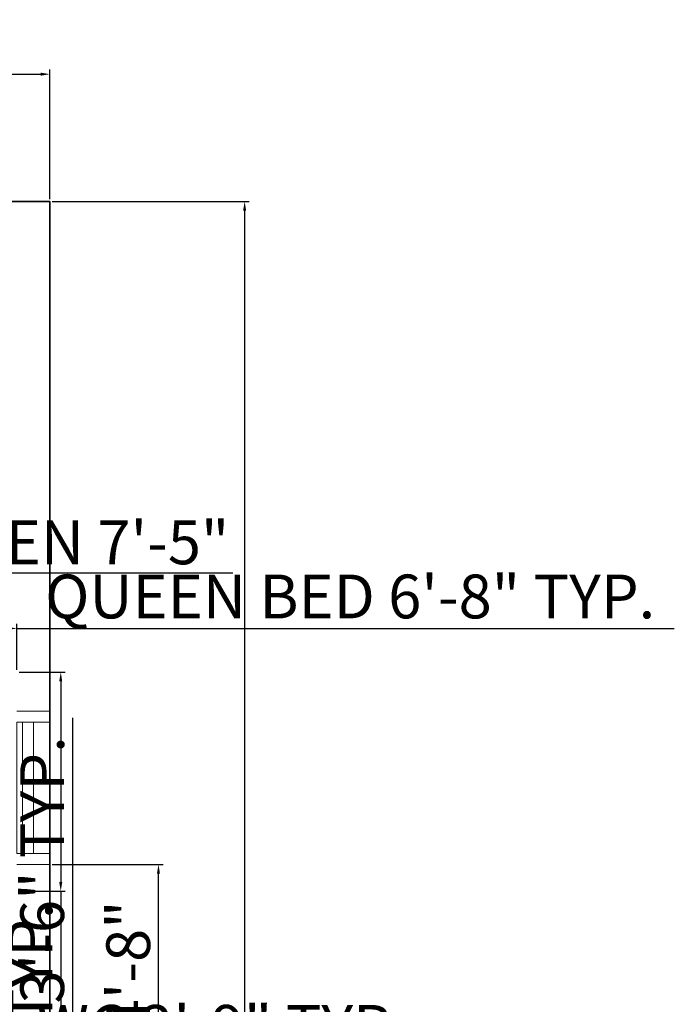
# Model space of a CAD drawing. Units: inches. Extents: x 2011 to 2548, y 530 to 1188.
# Tile 5 of 5: x 2368 to 2548, y 891 to 1161. Entities that reach past the tile are written whole.
import ezdxf

# ---------------------------------------------------------------- set-up
doc = ezdxf.new("R2010")
doc.units = ezdxf.units.IN
for name, color, linetype, lineweight in [('A-ANNO-DIMS', 2, 'Continuous', 18), ('A-GLAZ', 4, 'Continuous', 18), ('A-WALL', 7, 'Continuous', 35)]:
    doc.layers.add(name, color=color, linetype=linetype, lineweight=lineweight)
doc.styles.get("Standard").update_dxf_attribs({"font": 'arial.ttf'})
doc.dimstyles.new('ISO-25', dxfattribs={"dimtxt": 12, "dimasz": 2.5, "dimexe": 1.25, "dimexo": 0.625, "dimtad": 1, "dimdec": 1, "dimlunit": 3, "dimtxsty": 'Standard', "dimcen": 2.5, "dimadec": 0, "dimazin": 0, "dimtfac": 1, "dimtdec": 1, "dimtmove": 0, "dimatfit": 3, "dimfxl": 1, "dimarcsym": 0})

# ---------------------------------------------------------------- blocks, each defined once
blk = doc.blocks.new('*D12')
at = {"layer": 'A-ANNO-DIMS', "color": 0, "lineweight": -2, "transparency": 16777216}
for p, q in [((2076.53, 1111.98), (2076.53, 1147.49)), ((2376.53, 1111.98), (2376.53, 1147.49)), ((2079.03, 1146.24), (2374.03, 1146.24))]:
    blk.add_line(p, q, dxfattribs=at)
at = {"layer": 'A-ANNO-DIMS', "color": 0, "transparency": 16777216}
for points in [[(2079.03, 1146.66), (2079.03, 1145.82), (2076.53, 1146.24)], [(2374.03, 1146.66), (2374.03, 1145.82), (2376.53, 1146.24)]]:
    blk.add_solid(points, dxfattribs=at)
at = {"layer": 'Defpoints', "color": 0, "transparency": 16777216}
for p in [(2376.53, 1146.24), (2076.53, 1111.36), (2376.53, 1111.36)]:
    blk.add_point(p, dxfattribs=at)
at = {"layer": 'A-ANNO-DIMS', "color": 0, "transparency": 16777216, "insert": (2226.53, 1152.99), "char_height": 12, "attachment_point": 5}
blk.add_mtext("25'", dxfattribs=at)
blk = doc.blocks.new('*D13')
at = {"layer": 'A-ANNO-DIMS', "color": 0, "lineweight": -2, "transparency": 16777216}
for p, q in [((2377.15, 1111.36), (2431.21, 1111.36)), ((2429.96, 1108.86), (2429.96, 573.86)), ((2377.15, 571.36), (2431.21, 571.36))]:
    blk.add_line(p, q, dxfattribs=at)
at = {"layer": 'A-ANNO-DIMS', "color": 0, "transparency": 16777216}
for points in [[(2429.55, 1108.86), (2430.38, 1108.86), (2429.96, 1111.36)], [(2429.55, 573.86), (2430.38, 573.86), (2429.96, 571.36)]]:
    blk.add_solid(points, dxfattribs=at)
at = {"layer": 'Defpoints', "color": 0, "transparency": 16777216}
for p in [(2376.53, 1111.36), (2376.53, 571.36), (2429.96, 571.36)]:
    blk.add_point(p, dxfattribs=at)
at = {"layer": 'A-ANNO-DIMS', "color": 0, "transparency": 16777216, "insert": (2423.24, 841.36), "char_height": 12, "attachment_point": 5, "rotation": 90}
blk.add_mtext("45'", dxfattribs=at)
blk = doc.blocks.new('WIN-36IN')
for p, q in [((0, 42), (9, 42)), ((0, 3), (0, 39)), ((0, 39), (9, 39)), ((1.5, 39), (1.5, 3)), ((4.5, 39), (4.5, 3)), ((9, 39), (9, 3)), ((9, 3), (0, 3)), ((9, 0), (0, 0))]:
    blk.add_line(p, q)
blk = doc.blocks.new('*D17')
at = {"layer": 'A-ANNO-DIMS', "color": 0, "lineweight": -2, "transparency": 16777216}
for p, q in [((2382.83, 784.45), (2382.83, 969.85)), ((2377.15, 784.45), (2384.08, 784.45)), ((2382.83, 744.95), (2382.83, 781.95)), ((2377.15, 742.45), (2384.08, 742.45))]:
    blk.add_line(p, q, dxfattribs=at)
at = {"layer": 'A-ANNO-DIMS', "color": 0, "transparency": 16777216}
for points in [[(2382.41, 781.95), (2383.24, 781.95), (2382.83, 784.45)], [(2382.41, 744.95), (2383.24, 744.95), (2382.83, 742.45)]]:
    blk.add_solid(points, dxfattribs=at)
at = {"layer": 'Defpoints', "color": 0, "transparency": 16777216}
for p in [(2376.53, 784.45), (2382.83, 784.45), (2376.53, 742.45)]:
    blk.add_point(p, dxfattribs=at)
at = {"layer": 'A-ANNO-DIMS', "color": 0, "transparency": 16777216, "insert": (2375.99, 878.4), "char_height": 12, "attachment_point": 5, "rotation": 90}
blk.add_mtext('WINDOW W1 3\'-6" TYP.', dxfattribs=at)
blk = doc.blocks.new('*D23')
at = {"layer": 'A-ANNO-DIMS', "color": 0, "lineweight": -2, "transparency": 16777216}
for p, q in [((2334.48, 872.46), (2334.48, 878.04)), ((2367.53, 872.46), (2367.53, 878.04)), ((2336.98, 876.79), (2365.03, 876.79)), ((2367.53, 876.79), (2477.5, 876.79))]:
    blk.add_line(p, q, dxfattribs=at)
at = {"layer": 'A-ANNO-DIMS', "color": 0, "transparency": 16777216}
for points in [[(2336.98, 877.21), (2336.98, 876.38), (2334.48, 876.79)], [(2365.03, 877.21), (2365.03, 876.38), (2367.53, 876.79)]]:
    blk.add_solid(points, dxfattribs=at)
at = {"layer": 'Defpoints', "color": 0, "transparency": 16777216}
for p in [(2367.53, 876.79), (2334.48, 871.84), (2367.53, 871.84)]:
    blk.add_point(p, dxfattribs=at)
at = {"layer": 'A-ANNO-DIMS', "color": 0, "transparency": 16777216, "insert": (2423.76, 883.62), "char_height": 12, "attachment_point": 5}
blk.add_mtext('WC 2\'-9" TYP.', dxfattribs=at)
blk = doc.blocks.new('*D25')
at = {"layer": 'A-ANNO-DIMS', "color": 0, "lineweight": -2, "transparency": 16777216}
for p, q in [((2287.53, 982.98), (2287.53, 995.61)), ((2290.03, 994.36), (2365.03, 994.36)), ((2367.53, 982.98), (2367.53, 995.61)), ((2367.53, 994.36), (2547.8, 994.36))]:
    blk.add_line(p, q, dxfattribs=at)
at = {"layer": 'A-ANNO-DIMS', "color": 0, "transparency": 16777216}
for points in [[(2290.03, 994.78), (2290.03, 993.94), (2287.53, 994.36)], [(2365.03, 994.78), (2365.03, 993.94), (2367.53, 994.36)]]:
    blk.add_solid(points, dxfattribs=at)
at = {"layer": 'Defpoints', "color": 0, "transparency": 16777216}
for p in [(2367.53, 994.36), (2287.53, 982.36), (2367.53, 982.36)]:
    blk.add_point(p, dxfattribs=at)
at = {"layer": 'A-ANNO-DIMS', "color": 0, "transparency": 16777216, "insert": (2458.91, 1001.56), "char_height": 12, "attachment_point": 5}
blk.add_mtext('QUEEN BED 6\'-8" TYP.', dxfattribs=at)
blk = doc.blocks.new('*D26')
at = {"layer": 'A-ANNO-DIMS', "color": 0, "lineweight": -2, "transparency": 16777216}
for p, q in [((2368.15, 982.36), (2380.78, 982.36)), ((2379.53, 979.86), (2379.53, 924.86)), ((2368.15, 922.36), (2380.78, 922.36)), ((2379.53, 922.36), (2379.53, 845.46))]:
    blk.add_line(p, q, dxfattribs=at)
at = {"layer": 'A-ANNO-DIMS', "color": 0, "transparency": 16777216}
for points in [[(2379.11, 979.86), (2379.94, 979.86), (2379.53, 982.36)], [(2379.11, 924.86), (2379.94, 924.86), (2379.53, 922.36)]]:
    blk.add_solid(points, dxfattribs=at)
at = {"layer": 'Defpoints', "color": 0, "transparency": 16777216}
for p in [(2367.53, 982.36), (2367.53, 922.36), (2379.53, 922.36)]:
    blk.add_point(p, dxfattribs=at)
at = {"layer": 'A-ANNO-DIMS', "color": 0, "transparency": 16777216, "insert": (2372.78, 882.66), "char_height": 12, "attachment_point": 5, "rotation": 90}
blk.add_mtext('5\'-0" TYP.', dxfattribs=at)
blk = doc.blocks.new('*D29')
at = {"layer": 'A-ANNO-DIMS', "color": 0, "lineweight": -2, "transparency": 16777216}
for p, q in [((2224.2, 1022.31), (2224.2, 1008.31)), ((2313.39, 1022.31), (2313.39, 1008.31)), ((2226.7, 1009.56), (2310.89, 1009.56)), ((2313.39, 1009.56), (2426.74, 1009.56))]:
    blk.add_line(p, q, dxfattribs=at)
at = {"layer": 'A-ANNO-DIMS', "color": 0, "transparency": 16777216}
for points in [[(2226.7, 1009.97), (2226.7, 1009.14), (2224.2, 1009.56)], [(2310.89, 1009.97), (2310.89, 1009.14), (2313.39, 1009.56)]]:
    blk.add_solid(points, dxfattribs=at)
at = {"layer": 'Defpoints', "color": 0, "transparency": 16777216}
for p in [(2224.2, 1022.94), (2313.39, 1022.94), (2313.39, 1009.56)]:
    blk.add_point(p, dxfattribs=at)
at = {"layer": 'A-ANNO-DIMS', "color": 0, "transparency": 16777216, "insert": (2371.32, 1016.39), "char_height": 12, "attachment_point": 5}
blk.add_mtext('KITCHEN 7\'-5"', dxfattribs=at)
blk = doc.blocks.new('*D52')
at = {"layer": 'A-ANNO-DIMS', "color": 0, "lineweight": -2, "transparency": 16777216}
for p, q in [((2377.15, 929.66), (2407.58, 929.66)), ((2406.33, 876.31), (2406.33, 927.16)), ((2377.15, 873.81), (2407.58, 873.81))]:
    blk.add_line(p, q, dxfattribs=at)
at = {"layer": 'A-ANNO-DIMS', "color": 0, "transparency": 16777216}
for points in [[(2405.91, 927.16), (2406.74, 927.16), (2406.33, 929.66)], [(2405.91, 876.31), (2406.74, 876.31), (2406.33, 873.81)]]:
    blk.add_solid(points, dxfattribs=at)
at = {"layer": 'Defpoints', "color": 0, "transparency": 16777216}
for p in [(2376.53, 929.66), (2406.33, 929.66), (2376.53, 873.81)]:
    blk.add_point(p, dxfattribs=at)
at = {"layer": 'A-ANNO-DIMS', "color": 0, "transparency": 16777216, "insert": (2399.58, 901.74), "char_height": 12, "attachment_point": 5, "rotation": 90}
blk.add_mtext('4\'-8"', dxfattribs=at)

msp = doc.modelspace()

# ---------------------------------------------------------------- linework, layer by layer
at = {"layer": 'A-WALL'}
msp.add_lwpolyline([(2076.53, 1060.36), (2076.53, 571.36), (2376.53, 571.36), (2376.53, 1111.36), (2076.53, 1111.36), (2076.53, 1096.36)], dxfattribs=at)

# ---------------------------------------------------------------- block references
at = {"layer": 'A-GLAZ'}
msp.add_blockref('WIN-36IN', (2367.53, 929.66), dxfattribs=at)

# ---------------------------------------------------------------- dimensions: what is measured, and where the dimension line sits
at = {"layer": 'A-ANNO-DIMS'}
dim = msp.add_linear_dim(base=(2376.53, 1146.24), p1=(2076.53, 1111.36), p2=(2376.53, 1111.36), dimstyle='ISO-25', override={"dimclrd": 0, "dimclre": 0, "dimclrt": 0}, dxfattribs=at)
dim.commit()
dim.dimension.update_dxf_attribs({"geometry": '*D12', "text_midpoint": (2226.53, 1152.99)})
for base, p1, p2, override, picture, middle in [((2429.96, 571.36), (2376.53, 1111.36), (2376.53, 571.36), {"dimclrd": 0, "dimclre": 0, "dimclrt": 0}, '*D13', (2423.24, 841.36)), ((2406.327, 929.6645), (2376.527, 873.8101), (2376.527, 929.6645), {"dimdec": 1, "dimlfac": 1, "dimrnd": 0, "dimzin": 1, "dimdsep": 46, "dimlunit": 4, "dimfrac": 2}, '*D52', (2399.5751, 901.7373))]:
    dim = msp.add_linear_dim(base=base, p1=p1, p2=p2, angle=90, dimstyle='ISO-25', override=override, dxfattribs=at)
    dim.commit()
    dim.dimension.update_dxf_attribs({"geometry": picture, "text_midpoint": middle})
for base, p1, p2, text, picture, middle in [((2367.53, 994.36), (2287.53, 982.36), (2367.53, 982.36), 'QUEEN BED <> TYP.', '*D25', (2458.91, 1001.56)), ((2313.39, 1009.56), (2224.2, 1022.94), (2313.39, 1022.94), 'KITCHEN <>', '*D29', (2371.32, 1016.39)), ((2367.527, 876.7924), (2334.4807, 871.8355), (2367.527, 871.8355), 'WC <> TYP.', '*D23', (2423.7639, 883.622))]:
    dim = msp.add_linear_dim(base=base, p1=p1, p2=p2, text=text, dimstyle='ISO-25', override={"dimdec": 1, "dimlfac": 1, "dimrnd": 0, "dimzin": 1, "dimdsep": 46, "dimlunit": 4, "dimfrac": 2}, dxfattribs=at)
    dim.commit()
    dim.dimension.update_dxf_attribs({"geometry": picture, "text_midpoint": middle})
for base, p1, p2, angle, text, picture, middle in [((2379.53, 922.36), (2367.53, 982.36), (2367.53, 922.36), 270, '<> TYP.', '*D26', (2372.78, 882.66)), ((2382.83, 784.45), (2376.53, 742.45), (2376.53, 784.45), 90, 'WINDOW W1 <> TYP.', '*D17', (2375.99, 878.4))]:
    dim = msp.add_linear_dim(base=base, p1=p1, p2=p2, angle=angle, text=text, dimstyle='ISO-25', override={"dimdec": 1, "dimlfac": 1, "dimrnd": 0, "dimzin": 1, "dimdsep": 46, "dimlunit": 4, "dimfrac": 2}, dxfattribs=at)
    dim.commit()
    dim.dimension.update_dxf_attribs({"geometry": picture, "text_midpoint": middle})

doc.saveas('drawing.dxf')
